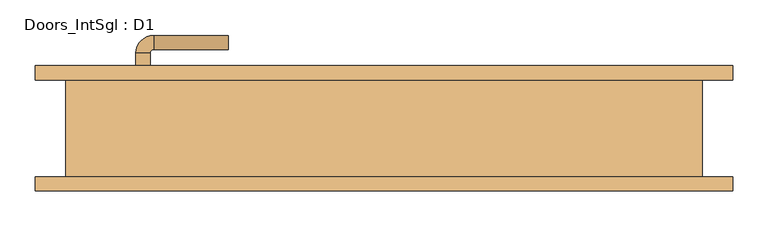
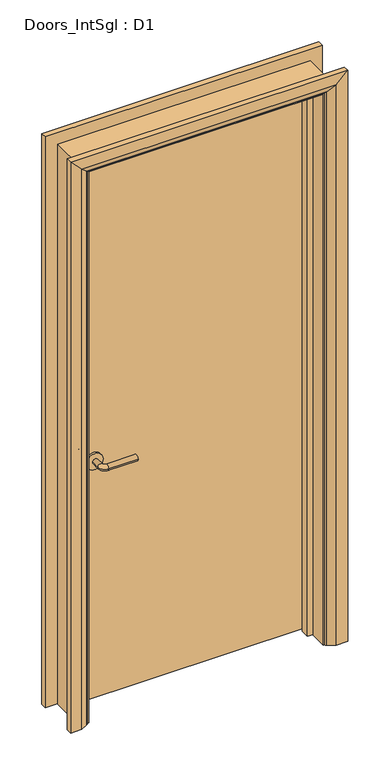
"""IFC4 building model written with IfcOpenShell, lengths in millimetres: door geometry, Doors_IntSgl : D1."""

from ifc_helpers import new_model, si_unit, point, frame, frame_2d, origin, place, context, project, spatial, polyline, circle_curve, ellipse_curve, trimmed, segment, composite_curve, outline, extrude, faceted_brep, source, transform, mapped, element, save
from ifc_brep_helpers import plane_surface, cylinder_surface, revolved_surface, advanced_brep


def doors_intsgl_d1_0ae72840(model_context):
    return source(origin(), model_context, "Body", "SolidModel", [
        advanced_brep(
        [(-350.2, 22.58, 900.0), (-330.2, 22.58, 900.0), (-330.2, -7.42, 900.0), (-350.2, -7.42, 900.0), (-325.2, -12.42, 900.0), (-325.2, -32.42, 900.0), (-220.2, -32.42, 900.0), (-220.2, -12.42, 900.0)],
        [
            (0, 1, circle_curve(frame((-340.2, 22.58, 900.0), z_axis=(0.0, 1.0, 0.0), x_axis=(1.0, 0.0, 0.0)), 10.0)),
            (1, 0, circle_curve(frame((-340.2, 22.58, 900.0), z_axis=(0.0, 1.0, 0.0), x_axis=(1.0, 0.0, 0.0)), 10.0)),
            (1, 2),
            (2, 3, circle_curve(frame((-340.2, -7.42, 900.0), z_axis=(0.0, 1.0, 0.0), x_axis=(1.0, 0.0, 0.0)), 10.0)),
            (3, 0),
            (3, 2, circle_curve(frame((-340.2, -7.42, 900.0), z_axis=(0.0, 1.0, 0.0), x_axis=(1.0, 0.0, 0.0)), 10.0)),
            (4, 5, circle_curve(frame((-325.2, -22.42, 900.0), z_axis=(-1.0, 0.0, 0.0), x_axis=(0.0, 1.0, 0.0)), 10.0)),
            (5, 3, circle_curve(frame((-325.2, -7.42, 900.0), z_axis=(0.0, 0.0, -1.0), x_axis=(-1.0, 0.0, 0.0)), 25.0)),
            (2, 4, circle_curve(frame((-325.2, -7.42, 900.0), z_axis=(0.0, 0.0, 1.0), x_axis=(-1.0, 0.0, 0.0)), 5.0)),
            (5, 4, circle_curve(frame((-325.2, -22.42, 900.0), z_axis=(-1.0, 0.0, 0.0), x_axis=(0.0, 1.0, 0.0)), 10.0)),
            (6, 7, circle_curve(frame((-220.2, -22.42, 900.0), z_axis=(1.0, 0.0, 0.0), x_axis=(0.0, 1.0, 0.0)), 10.0)),
            (7, 6, circle_curve(frame((-220.2, -22.42, 900.0), z_axis=(1.0, 0.0, 0.0), x_axis=(0.0, 1.0, 0.0)), 10.0)),
            (4, 7),
            (6, 5),
        ],
        [
            plane_surface(frame((-340.2, 22.58, 900.0), z_axis=(0.0, 1.0, 0.0), x_axis=(0.0, 0.0, 1.0))),
            cylinder_surface(frame((-340.2, 22.58, 900.0), z_axis=(0.0, 1.0, 0.0), x_axis=(1.0, 0.0, 0.0)), 10.0),
            revolved_surface(trimmed(ellipse_curve(frame((-340.2, -7.42, 900.0), z_axis=(0.0, -1.0, 0.0), x_axis=(1.0, 0.0, 0.0)), 10.0, 10.0), [point((-350.2, -7.42, 900.0))], [point((-330.2, -7.42, 900.0))], True, "CARTESIAN"), (-325.2, -7.42, 900.0), (0.0, 0.0, -1.0)),
            revolved_surface(trimmed(ellipse_curve(frame((-340.2, -7.42, 900.0), z_axis=(0.0, -1.0, 0.0), x_axis=(1.0, 0.0, 0.0)), 10.0, 10.0), [point((-330.2, -7.42, 900.0))], [point((-350.2, -7.42, 900.0))], True, "CARTESIAN"), (-325.2, -7.42, 900.0), (0.0, 0.0, -1.0)),
            plane_surface(frame((-220.2, -22.42, 900.0), z_axis=(1.0, 0.0, 0.0), x_axis=(0.0, 0.0, 1.0))),
            cylinder_surface(frame((-325.2, -22.42, 900.0), z_axis=(-1.0, 0.0, 0.0), x_axis=(0.0, 1.0, 0.0)), 10.0),
        ],
        [
            (0, [[1, 2]]),
            (1, [[3, 4, 5, -2]]),
            (1, [[-5, 6, -3, -1]]),
            (2, [[7, 8, -4, 9]]),
            (3, [[10, -9, -6, -8]]),
            (4, [[11, 12]]),
            (5, [[13, -11, 14, -7]]),
            (5, [[-14, -12, -13, -10]]),
        ],
    ),
        extrude(outline(composite_curve([segment(trimmed(circle_curve(frame_2d((900.0, -342.7)), 30.0), [point((900.0, -372.7))], [point((900.0, -312.7))], False, "CARTESIAN"), True, "CONTINUOUS"), segment(trimmed(circle_curve(frame_2d((900.0, -342.7)), 30.0), [point((900.0, -312.7))], [point((900.0, -372.7))], False, "CARTESIAN"), True, "CONTINUOUS")], self_intersect=False)), frame((0.0, 22.58, 0.0), z_axis=(0.0, 1.0, 0.0), x_axis=(0.0, 0.0, 1.0)), (0.0, 0.0, 1.0), 8.0),
        advanced_brep(
        [(-350.2, 76.58, 900.0), (-330.2, 76.58, 900.0), (-350.2, 106.58, 900.0), (-330.2, 106.58, 900.0), (-325.2, 111.58, 900.0), (-325.2, 131.58, 900.0), (-220.2, 131.58, 900.0), (-220.2, 111.58, 900.0)],
        [
            (0, 1, circle_curve(frame((-340.2, 76.58, 900.0), z_axis=(0.0, -1.0, 0.0), x_axis=(1.0, 0.0, 0.0)), 10.0)),
            (1, 0, circle_curve(frame((-340.2, 76.58, 900.0), z_axis=(0.0, -1.0, 0.0), x_axis=(1.0, 0.0, 0.0)), 10.0)),
            (0, 2),
            (2, 3, circle_curve(frame((-340.2, 106.58, 900.0), z_axis=(0.0, -1.0, 0.0), x_axis=(1.0, 0.0, 0.0)), 10.0)),
            (3, 1),
            (3, 2, circle_curve(frame((-340.2, 106.58, 900.0), z_axis=(0.0, -1.0, 0.0), x_axis=(1.0, 0.0, 0.0)), 10.0)),
            (4, 3, circle_curve(frame((-325.2, 106.58, 900.0), z_axis=(0.0, 0.0, 1.0), x_axis=(-1.0, 0.0, 0.0)), 5.0)),
            (2, 5, circle_curve(frame((-325.2, 106.58, 900.0), z_axis=(0.0, 0.0, -1.0), x_axis=(-1.0, 0.0, 0.0)), 25.0)),
            (5, 4, circle_curve(frame((-325.2, 121.58, 900.0), z_axis=(-1.0, 0.0, 0.0), x_axis=(0.0, -1.0, 0.0)), 10.0)),
            (4, 5, circle_curve(frame((-325.2, 121.58, 900.0), z_axis=(-1.0, 0.0, 0.0), x_axis=(0.0, -1.0, 0.0)), 10.0)),
            (6, 7, circle_curve(frame((-220.2, 121.58, 900.0), z_axis=(1.0, 0.0, 0.0), x_axis=(0.0, -1.0, 0.0)), 10.0)),
            (7, 6, circle_curve(frame((-220.2, 121.58, 900.0), z_axis=(1.0, 0.0, 0.0), x_axis=(0.0, -1.0, 0.0)), 10.0)),
            (5, 6),
            (7, 4),
        ],
        [
            plane_surface(frame((-340.2, 76.58, 900.0), z_axis=(0.0, -1.0, 0.0), x_axis=(0.0, 0.0, 1.0))),
            cylinder_surface(frame((-340.2, 76.58, 900.0), z_axis=(0.0, -1.0, 0.0), x_axis=(1.0, 0.0, 0.0)), 10.0),
            revolved_surface(trimmed(ellipse_curve(frame((-340.2, 106.58, 900.0), z_axis=(0.0, -1.0, 0.0), x_axis=(1.0, 0.0, 0.0)), 10.0, 10.0), [point((-350.2, 106.58, 900.0))], [point((-330.2, 106.58, 900.0))], True, "CARTESIAN"), (-325.2, 106.58, 900.0), (0.0, 0.0, -1.0)),
            revolved_surface(trimmed(ellipse_curve(frame((-340.2, 106.58, 900.0), z_axis=(0.0, -1.0, 0.0), x_axis=(1.0, 0.0, 0.0)), 10.0, 10.0), [point((-330.2, 106.58, 900.0))], [point((-350.2, 106.58, 900.0))], True, "CARTESIAN"), (-325.2, 106.58, 900.0), (0.0, 0.0, -1.0)),
            plane_surface(frame((-220.2, 121.58, 900.0), z_axis=(1.0, 0.0, 0.0), x_axis=(0.0, 0.0, 1.0))),
            cylinder_surface(frame((-325.2, 121.58, 900.0), z_axis=(-1.0, 0.0, 0.0), x_axis=(0.0, -1.0, 0.0)), 10.0),
        ],
        [
            (0, [[1, 2]]),
            (1, [[-1, 3, 4, 5]]),
            (1, [[-2, -5, 6, -3]]),
            (2, [[7, -4, 8, 9]]),
            (3, [[-8, -6, -7, 10]]),
            (4, [[11, 12]]),
            (5, [[-9, 13, -12, 14]]),
            (5, [[-10, -14, -11, -13]]),
        ],
    ),
        extrude(outline(composite_curve([segment(trimmed(circle_curve(frame_2d((900.0, -342.7)), 30.0), [point((900.0, -372.7))], [point((900.0, -312.7))], False, "CARTESIAN"), True, "CONTINUOUS"), segment(trimmed(circle_curve(frame_2d((900.0, -342.7)), 30.0), [point((900.0, -312.7))], [point((900.0, -372.7))], False, "CARTESIAN"), True, "CONTINUOUS")], self_intersect=False)), frame((0.0, 68.58, 0.0), z_axis=(0.0, 1.0, 0.0), x_axis=(0.0, 0.0, 1.0)), (0.0, 0.0, 1.0), 8.0),
        extrude(outline(polyline([(415.2, 30.58), (-415.2, 30.58), (-415.2, 68.58), (415.2, 68.58), (415.2, 30.58)])), frame((0.0, 0.0, 8.0), z_axis=(0.0, 0.0, 1.0), x_axis=(1.0, 0.0, 0.0)), (0.0, 0.0, 1.0), 2060.0),
        advanced_brep(
        [(492.2, 88.58, 0.0), (492.2, 68.58, 0.0), (422.2, 68.58, 0.0), (426.2, 74.58, 0.0), (452.2, 88.58, 0.0), (492.2, 88.58, 2145.0), (492.2, 68.58, 2145.0), (-492.2, 68.58, 2145.0), (-492.2, 68.58, 0.0), (-422.2, 68.58, 0.0), (-422.2, 68.58, 2075.0), (422.2, 68.58, 2075.0), (426.2, 74.58, 2079.0), (452.2, 88.58, 2105.0), (-452.2, 88.58, 2105.0), (-452.2, 88.58, 0.0), (-492.2, 88.58, 0.0), (-492.2, 88.58, 2145.0), (-426.2, 74.58, 0.0), (-426.2, 74.58, 2079.0)],
        [
            (0, 1),
            (1, 2),
            (2, 3, circle_curve(frame((430.2, 67.58, 0.0), z_axis=(0.0, 0.0, -1.0), x_axis=(1.0, 0.0, 0.0)), 8.0622577)),
            (3, 4),
            (4, 0),
            (0, 5),
            (5, 6),
            (6, 1),
            (6, 7),
            (7, 8),
            (8, 9),
            (9, 10),
            (10, 11),
            (11, 2),
            (11, 12, ellipse_curve(frame((430.2, 67.58, 2083.0), z_axis=(0.7071067811865475, 0.0, -0.7071067811865475), x_axis=(-0.7071067811865474, 0.0, -0.7071067811865476)), 11.4017543, 8.0622577)),
            (12, 3),
            (12, 13),
            (13, 4),
            (13, 14),
            (14, 15),
            (15, 16),
            (16, 17),
            (17, 5),
            (7, 17),
            (16, 8),
            (15, 18),
            (18, 9, circle_curve(frame((-430.2, 67.58, 0.0), z_axis=(0.0, 0.0, -1.0), x_axis=(-1.0, 0.0, 0.0)), 8.0622577)),
            (19, 10, ellipse_curve(frame((-430.2, 67.58, 2083.0), z_axis=(-0.7071067811865475, 0.0, -0.7071067811865475), x_axis=(-0.7071067811865474, 0.0, 0.7071067811865476)), 11.4017543, 8.0622577)),
            (18, 19),
            (14, 19),
            (19, 12),
        ],
        [
            plane_surface(frame((422.2, 68.58, 0.0), z_axis=(0.0, 0.0, -1.0), x_axis=(0.0, -1.0, 0.0))),
            plane_surface(frame((492.2, 88.58, 0.0), z_axis=(1.0, 0.0, 0.0), x_axis=(0.0, 0.0, 1.0))),
            plane_surface(frame((492.2, 68.58, 0.0), z_axis=(0.0, -1.0, 0.0), x_axis=(0.0, 0.0, 1.0))),
            cylinder_surface(frame((430.2, 67.58, 0.0), z_axis=(0.0, 0.0, -1.0), x_axis=(1.0, 0.0, 0.0)), 8.0622577),
            plane_surface(frame((426.2, 74.58, 0.0), z_axis=(-0.4740998230350126, 0.880471099922178, 0.0), x_axis=(0.0, 0.0, 1.0))),
            plane_surface(frame((452.2, 88.58, 0.0), z_axis=(0.0, 1.0, 0.0), x_axis=(0.0, 0.0, 1.0))),
            plane_surface(frame((-492.2, 88.58, 2145.0), z_axis=(-1.0, 0.0, 0.0), x_axis=(0.0, 0.0, -1.0))),
            plane_surface(frame((-422.2, 68.58, 0.0), z_axis=(0.0, 0.0, -1.0), x_axis=(0.0, -1.0, 0.0))),
            cylinder_surface(frame((-430.2, 67.58, 2075.0), z_axis=(0.0, 0.0, 1.0), x_axis=(-1.0, 0.0, 0.0)), 8.0622577),
            plane_surface(frame((-426.2, 74.58, 2079.0), z_axis=(0.47409982303501824, 0.8804710999221749, 0.0), x_axis=(0.0, 0.0, -1.0))),
            plane_surface(frame((492.2, 88.58, 2145.0), z_axis=(0.0, 0.0, 1.0), x_axis=(-1.0, 0.0, 0.0))),
            cylinder_surface(frame((422.2, 67.58, 2083.0), z_axis=(1.0, 0.0, 0.0), x_axis=(0.0, 0.0, 1.0)), 8.0622577),
            plane_surface(frame((426.2, 74.58, 2079.0), z_axis=(0.0, 0.8804710999221764, -0.4740998230350154), x_axis=(-1.0, 0.0, 0.0))),
        ],
        [
            (0, [[1, 2, 3, 4, 5]]),
            (1, [[-1, 6, 7, 8]]),
            (2, [[-2, -8, 9, 10, 11, 12, 13, 14]]),
            (3, [[-3, -14, 15, 16]]),
            (4, [[-4, -16, 17, 18]]),
            (5, [[-5, -18, 19, 20, 21, 22, 23, -6]]),
            (6, [[24, -22, 25, -10]]),
            (7, [[-21, 26, 27, -11, -25]]),
            (8, [[28, -12, -27, 29]]),
            (9, [[30, -29, -26, -20]]),
            (10, [[-7, -23, -24, -9]]),
            (11, [[-15, -13, -28, 31]]),
            (12, [[-17, -31, -30, -19]]),
        ],
    ),
        extrude(outline(polyline([(0.0, -417.2), (0.0, -398.2), (2051.0, -398.2), (2051.0, 398.2), (0.0, 398.2), (0.0, 417.2), (2070.0, 417.2), (2070.0, -417.2), (0.0, -417.2)])), frame((0.0, -3.42, 0.0), z_axis=(0.0, 1.0, 0.0), x_axis=(0.0, 0.0, 1.0)), (0.0, 0.0, 1.0), 32.0),
        advanced_brep(
        [(-492.2, -88.58, 0.0), (-492.2, -68.58, 0.0), (-422.2, -68.58, 0.0), (-426.2, -74.58, 0.0), (-452.2, -88.58, 0.0), (-492.2, -88.58, 2145.0), (-492.2, -68.58, 2145.0), (-422.2, -68.58, 2075.0), (-426.2, -74.58, 2079.0), (-452.2, -88.58, 2105.0), (492.2, -88.58, 0.0), (452.2, -88.58, 0.0), (426.2, -74.58, 0.0), (422.2, -68.58, 0.0), (492.2, -68.58, 0.0), (492.2, -88.58, 2145.0), (452.2, -88.58, 2105.0), (426.2, -74.58, 2079.0), (422.2, -68.58, 2075.0), (492.2, -68.58, 2145.0)],
        [
            (0, 1),
            (1, 2),
            (2, 3, circle_curve(frame((-430.2, -67.58, 0.0), z_axis=(0.0, 0.0, -1.0), x_axis=(-1.0, 0.0, 0.0)), 8.0622577)),
            (3, 4),
            (4, 0),
            (0, 5),
            (5, 6),
            (6, 1),
            (6, 7),
            (7, 2),
            (7, 8, ellipse_curve(frame((-430.2, -67.58, 2083.0), z_axis=(-0.7071067811865475, 0.0, -0.7071067811865475), x_axis=(0.7071067811865474, 0.0, -0.7071067811865476)), 11.4017543, 8.0622577)),
            (8, 3),
            (8, 9),
            (9, 4),
            (9, 5),
            (10, 11),
            (11, 12),
            (12, 13, circle_curve(frame((430.2, -67.58, 0.0), z_axis=(0.0, 0.0, -1.0), x_axis=(1.0, 0.0, 0.0)), 8.0622577)),
            (13, 14),
            (14, 10),
            (15, 16),
            (16, 11),
            (10, 15),
            (16, 17),
            (17, 12),
            (17, 18, ellipse_curve(frame((430.2, -67.58, 2083.0), z_axis=(0.7071067811865475, 0.0, -0.7071067811865475), x_axis=(0.7071067811865474, 0.0, 0.7071067811865476)), 11.4017543, 8.0622577)),
            (18, 13),
            (18, 19),
            (19, 14),
            (19, 15),
            (5, 15),
            (19, 6),
            (18, 7),
            (17, 8),
            (16, 9),
        ],
        [
            plane_surface(frame((-422.2, -141.3810989, 0.0), z_axis=(0.0, 0.0, -1.0), x_axis=(1.0, 0.0, 0.0))),
            plane_surface(frame((-492.2, -88.58, 0.0), z_axis=(-1.0, 0.0, 0.0), x_axis=(0.0, 0.0, 1.0))),
            plane_surface(frame((-492.2, -68.58, 0.0), z_axis=(0.0, 1.0, 0.0), x_axis=(0.0, 0.0, 1.0))),
            cylinder_surface(frame((-430.2, -67.58, 0.0), z_axis=(0.0, 0.0, -1.0), x_axis=(-1.0, 0.0, 0.0)), 8.0622577),
            plane_surface(frame((-426.2, -74.58, 0.0), z_axis=(0.4740998230350183, -0.8804710999221749, 0.0), x_axis=(0.0, 0.0, 1.0))),
            plane_surface(frame((-452.2, -88.58, 0.0), z_axis=(0.0, -1.0, 0.0), x_axis=(0.0, 0.0, 1.0))),
            plane_surface(frame((422.2, -141.3810989, 0.0), z_axis=(0.0, 0.0, -1.0), x_axis=(-1.0, 0.0, 0.0))),
            plane_surface(frame((452.2, -88.58, 2105.0), z_axis=(0.0, -1.0, 0.0), x_axis=(0.0, 0.0, -1.0))),
            plane_surface(frame((426.2, -74.58, 2079.0), z_axis=(-0.4740998230350183, -0.8804710999221749, 0.0), x_axis=(0.0, 0.0, -1.0))),
            cylinder_surface(frame((430.2, -67.58, 2075.0), z_axis=(0.0, 0.0, 1.0), x_axis=(1.0, 0.0, 0.0)), 8.0622577),
            plane_surface(frame((492.2, -68.58, 2145.0), z_axis=(0.0, 1.0, 0.0), x_axis=(0.0, 0.0, -1.0))),
            plane_surface(frame((492.2, -88.58, 2145.0), z_axis=(1.0, 0.0, 0.0), x_axis=(0.0, 0.0, -1.0))),
            plane_surface(frame((-492.2, -88.58, 2145.0), z_axis=(0.0, 0.0, 1.0), x_axis=(1.0, 0.0, 0.0))),
            plane_surface(frame((-492.2, -68.58, 2145.0), z_axis=(0.0, 1.0, 0.0), x_axis=(1.0, 0.0, 0.0))),
            cylinder_surface(frame((-422.2, -67.58, 2083.0), z_axis=(-1.0, 0.0, 0.0), x_axis=(0.0, 0.0, 1.0)), 8.0622577),
            plane_surface(frame((-426.2, -74.58, 2079.0), z_axis=(0.0, -0.8804710999221749, -0.4740998230350183), x_axis=(1.0, 0.0, 0.0))),
            plane_surface(frame((-452.2, -88.58, 2105.0), z_axis=(0.0, -1.0, 0.0), x_axis=(1.0, 0.0, 0.0))),
        ],
        [
            (0, [[1, 2, 3, 4, 5]]),
            (1, [[-1, 6, 7, 8]]),
            (2, [[-2, -8, 9, 10]]),
            (3, [[-3, -10, 11, 12]]),
            (4, [[-4, -12, 13, 14]]),
            (5, [[-5, -14, 15, -6]]),
            (6, [[16, 17, 18, 19, 20]]),
            (7, [[21, 22, -16, 23]]),
            (8, [[24, 25, -17, -22]]),
            (9, [[26, 27, -18, -25]]),
            (10, [[28, 29, -19, -27]]),
            (11, [[30, -23, -20, -29]]),
            (12, [[-7, 31, -30, 32]]),
            (13, [[-9, -32, -28, 33]]),
            (14, [[-11, -33, -26, 34]]),
            (15, [[-13, -34, -24, 35]]),
            (16, [[-15, -35, -21, -31]]),
        ],
    ),
        faceted_brep([(-417.2, 68.58, 0.0), (-417.2, -68.58, 0.0), (-449.2, -68.58, 0.0), (-449.2, 68.58, 0.0), (-417.2, 68.58, 2070.0), (-417.2, -68.58, 2070.0), (-449.2, -68.58, 2102.0), (-449.2, 68.58, 2102.0), (417.2, 68.58, 0.0), (449.2, 68.58, 0.0), (449.2, -68.58, 0.0), (417.2, -68.58, 0.0), (417.2, 68.58, 2070.0), (449.2, 68.58, 2102.0), (449.2, -68.58, 2102.0), (417.2, -68.58, 2070.0)], [[[0, 1, 2, 3]], [[1, 0, 4, 5]], [[2, 1, 5, 6]], [[3, 2, 6, 7]], [[0, 3, 7, 4]], [[8, 9, 10, 11]], [[12, 13, 9, 8]], [[13, 14, 10, 9]], [[14, 15, 11, 10]], [[15, 12, 8, 11]], [[5, 4, 12, 15]], [[6, 5, 15, 14]], [[7, 6, 14, 13]], [[4, 7, 13, 12]]]),
    ])


if __name__ == "__main__":
    model = new_model("IFC4")
    model_context = context("Model", 3, world=origin())
    ifc_project = project(units=[si_unit("LENGTHUNIT", "METRE", prefix="MILLI")], contexts=[model_context])
    site = spatial("IfcSite", under=ifc_project)
    building = spatial("IfcBuilding", under=site)
    placement = place(None, origin())
    doors_intsgl_d1_shape = doors_intsgl_d1_0ae72840(model_context)
    element("IfcDoor", 1, ObjectType="Doors_IntSgl : D1", at=placement, inside=building, context=model_context, shape_type="MappedRepresentation", body=[
        mapped(doors_intsgl_d1_shape, transform((0.0, 0.0, 0.0), x_axis=(1.0, 0.0, 0.0), y_axis=(0.0, 1.0, 0.0), z_axis=(0.0, 0.0, 1.0))),
    ])
    save(model, "model.ifc")

# Revit data of these elements
# Type "Doors_IntSgl : D1"
#   Type Mark = "46"
#   Type Comments = "Internal Single"
#   Operation = "SingleSwingRight"
#   Manufacturer = "Revit"
#   Keynote = "L20"
#   Description = "Internal Single Door"
#   Analytic Construction = "Metal"
#   UnderCut = 8 mm
#   Tolerance = 2 mm
#   Thickness = 38 mm
#   Thermal Resistance (R) = 0.270117 (m²·K)/W
#   Structural Tolerance = 8 mm
#   StopDepth = 32 mm
#   Stop Thickness = 19 mm
#   Rough Width = 914.4 mm
#   Rough Height = 2110 mm
#   Height to Top Lock Rail = 1000 mm
#   Heat Transfer Coefficient (U) = 3.7021 W/(m²·K)
#   Handle Z Distance = 900 mm
#   Handle X Distance = 75 mm
#   Frame Thickness = 32 mm
#   Door Panel Width = 830.4 mm
#   Door Panel Thickness = 38 mm
#   Door Panel Offset = 0 mm
#   Height = 2110 mm
#   Width = 914.4 mm
#   Door Panel Height = 2060 mm
#   Architrave Setback = 5 mm
#   Vis - Ironmongery = yes
#   Material Ironmongery = Door - Handle
#   Material Frame = Door - Frame/Mullion (1)
#   Material Door = Door - Panel
#   Material Architrave = Door - Architrave
#   Visual Light Transmittance = 0
#   Solar Heat Gain Coefficient = 0
#   Function = (empty or 0)
#   Wall Closure = (empty or 0)
# Element 1 (IfcDoor, "Doors_IntSgl : D1")
#   Materials on its faces: "Door - Architrave", "Door - Handle", "Door - Frame/Mullion (1)", "Door - Panel"
# Materials
#   "Door - Handle": colour RGB 0 0 0, transparency 0, Keynote = "P21", Cost = 0
#   "Door - Frame/Mullion (1)": class "Wood", colour RGB 212 179 113, transparency 0, Keynote = "L20", Cost = 0
#   "Door - Panel": class "Wood", colour RGB 210 159 95, transparency 0, Keynote = "L20", Cost = 0
#   "Door - Architrave": class "Wood", colour RGB 154 90 5, transparency 0, Keynote = "P20", Cost = 0
